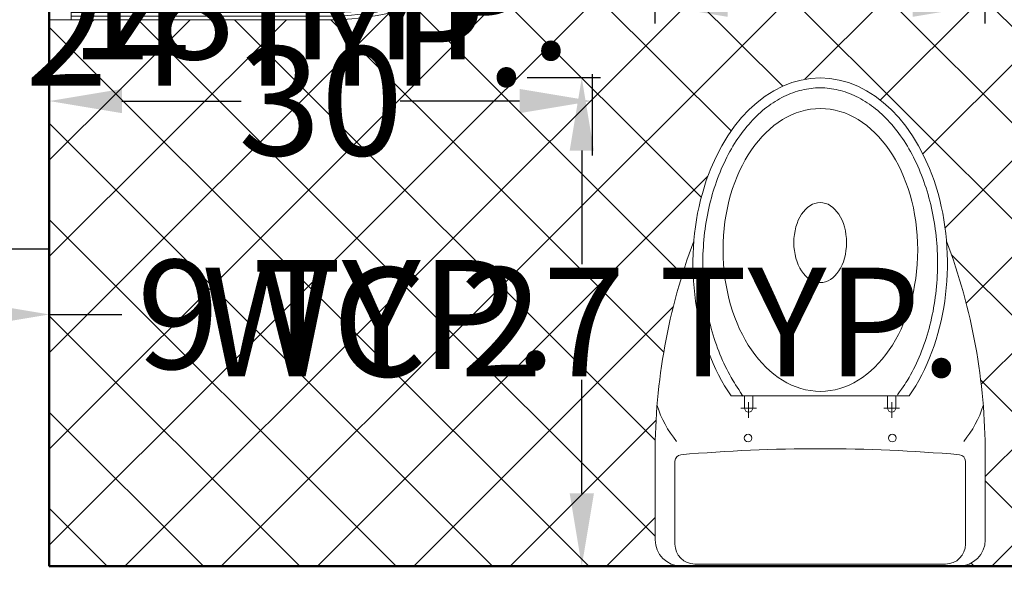
# Model space of a CAD drawing. Units: inches. Extents: x -466983 to 1020, y 324 to 318697.
# Tile 5 of 97: x 450 to 504, y 566 to 597. Entities that reach past the tile are written whole.
import ezdxf

# ---------------------------------------------------------------- set-up
doc = ezdxf.new("R2010")
doc.units = ezdxf.units.IN
doc.header["$MEASUREMENT"] = 0
for name, color, linetype, lineweight in [('A-ANNO-DIMS', 2, 'Continuous', 18), ('A-FLOR-FIXT', 9, 'Continuous', 18), ('A-FLOR-PATT', 252, 'Continuous', 13), ('A-GLAZ', 4, 'Continuous', 25), ('A-WALL', 7, 'Continuous', 50)]:
    doc.layers.add(name, color=color, linetype=linetype, lineweight=lineweight)
doc.styles.get("Standard").update_dxf_attribs({"font": 'arial.ttf'})
doc.dimstyles.get("Standard").update_dxf_attribs({"dimtxt": 6, "dimasz": 4, "dimexe": 3, "dimexo": 3, "dimgap": 0.09, "dimtad": 0, "dimtih": 1, "dimtoh": 1, "dimdec": 1, "dimzin": 0, "dimdsep": 46, "dimlunit": 3, "dimtxsty": 'Standard', "dimcen": 0.09, "dimadec": 0, "dimazin": 0, "dimtfac": 1, "dimtdec": 1, "dimtofl": 0, "dimtmove": 0, "dimatfit": 3, "dimfxl": 1, "dimtolj": 1, "dimtzin": 0, "dimarcsym": 0})

# ---------------------------------------------------------------- blocks, each defined once
blk = doc.blocks.new('Ventilator')
for p, q in [((1433.5927409432, 801.6799676286266), (1457.592740943201, 801.6799676286266)), ((1433.5927409432, 792.6799676286266), (1433.5927409432, 801.6799676286266)), ((1457.592740943201, 801.6799676286266), (1457.592740943201, 792.6799676286266)), ((1433.5927409432, 797.9799676286265), (1457.592740943201, 797.9799676286265)), ((1457.592740943201, 796.3799676286266), (1433.5927409432, 796.3799676286266)), ((1457.592740943201, 792.6799676286266), (1433.5927409432, 792.6799676286266))]:
    blk.add_line(p, q)
blk = doc.blocks.new('B1')
for p, q in [((0, 1300.000000000277), (693.3333333334303, 1300.000000000277)), ((0, 1.023182e-10), (0, 1300.000000000277)), ((52.00000000000727, 52.00000000000045), (52.00000000000727, 1300.000000000277)), ((52.00000000000727, 1291.33333333362), (693.3333333334303, 1291.33333333362)), ((52.00000000000727, 1282.666666666948), (693.3333333334303, 1282.666666666948)), ((0, 1248.000000000277), (693.3333333334303, 1248.000000000277)), ((21.99999999999818, 689.0000000001346), (21.99999999999818, 687.0000000001382)), ((140.3876720592416, 699.4289321882679), (154.4144116848583, 699.4289321882679)), ((208.8876720592416, 705.4289321882679), (153.4804125083301, 702.8756022550479)), ((1248.000000000174, 693.6609680139231), (1248.000000000174, 1.023182e-10)), ((1282.666666666846, 693.6609680139231), (1282.666666666846, 52.00000000010231)), ((1291.333333333514, 693.6609680139231), (1291.333333333517, 52.00000000010231)), ((1300.000000000182, 693.6609680139231), (1300.000000000182, 1.023182e-10)), ((21.99999999999818, 663.0000000001382), (21.99999999999818, 665.0000000001309)), ((140.3876720592416, 652.5710678120049), (154.4144116848583, 652.5710678120049)), ((208.8876720592416, 646.5710678120049), (153.5459520445456, 648.976381547378)), ((52.00000000001091, 52.00000000000045), (1300.000000000178, 52.00000000010231)), ((0, 4.547e-13), (1300.000000000182, 1.023182e-10))]:
    blk.add_line(p, q)
for points in [[(0, 775.000000000131), (0, 789.0000000001346), (8, 789.0000000001346)], [(8, 789.0000000001346), (8, 717.0000000001309)], [(8, 789.0000000001346), (27.99999999999818, 769.0000000001309), (27.99999999999818, 767.0000000001382)], [(0, 754.0000000001382), (0, 775.000000000131)], [(27.99999999999818, 767.0000000001382), (33.00000000000182, 767.0000000001382)], [(27.99999999999818, 767.0000000001382), (27.99999999999818, 753.0000000001345)], [(33.00000000000182, 767.0000000001382), (35, 769.0000000001309), (43, 769.0000000001309), (45.00000000000182, 767.0000000001382)], [(33.00000000000182, 767.0000000001382), (33.00000000000182, 753.0000000001345)], [(35, 765.0000000001345), (33.00000000000182, 762.0000000001346)], [(33.00000000000182, 758.0000000001346), (35, 756.0000000001346), (43, 756.0000000001346), (45.00000000000182, 758.0000000001346)], [(43, 769.0000000001309), (43, 765.0000000001345), (35, 765.0000000001345), (35, 769.0000000001309)], [(35, 756.0000000001346), (35, 753.0000000001345)], [(43, 765.0000000001345), (45.00000000000182, 763.0000000001382)], [(43, 756.0000000001346), (43, 753.0000000001345)], [(47, 767.0000000001382), (45.00000000000182, 767.0000000001382)], [(45.00000000000182, 767.0000000001382), (45.00000000000182, 753.0000000001345)], [(47, 739.0000000001382), (47, 767.0000000001382)], [(8, 717.0000000001309), (0, 717.0000000001309), (0, 754.0000000001382)], [(8, 717.0000000001309), (27.99999999999818, 737.0000000001346), (27.99999999999818, 739.0000000001382)], [(27.99999999999818, 739.0000000001382), (27.99999999999818, 753.0000000001345)], [(27.99999999999818, 739.0000000001382), (33.00000000000182, 739.0000000001382)], [(33.00000000000182, 739.0000000001382), (33.00000000000182, 753.0000000001345)], [(33.00000000000182, 748.0000000001382), (35, 750.0000000001346), (43, 750.0000000001346), (45.00000000000182, 748.0000000001382)], [(35, 741.0000000001346), (33.00000000000182, 744.0000000001345)], [(33.00000000000182, 739.0000000001382), (35, 737.0000000001346), (43, 737.0000000001346), (45.00000000000182, 739.0000000001382)], [(35, 750.0000000001346), (35, 753.0000000001345)], [(43, 737.0000000001346), (43, 741.0000000001346), (35, 741.0000000001346), (35, 737.0000000001346)], [(43, 750.0000000001346), (43, 753.0000000001345)], [(43, 741.0000000001346), (45.00000000000182, 743.0000000001346)], [(45.00000000000182, 739.0000000001382), (45.00000000000182, 753.0000000001345)], [(47, 739.0000000001382), (45.00000000000182, 739.0000000001382)], [(47, 728.0000000001345), (47, 739.0000000001382)], [(0, 687.0000000001382), (0, 699.0000000001382)], [(0, 699.0000000001382), (3, 699.0000000001382)], [(0, 665.0000000001309), (0, 687.0000000001382)], [(3, 699.0000000001382), (3, 676.0000000001346)], [(3, 699.0000000001382), (11, 690.0000000001382), (11, 687.0000000001382)], [(11, 687.0000000001382), (11, 676.0000000001346)], [(140.9999999999982, 687.0000000001382), (11, 687.0000000001382)], [(0, 653.0000000001309), (0, 665.0000000001309)], [(3, 653.0000000001309), (3, 676.0000000001346)], [(3, 653.0000000001309), (11, 662.000000000131), (11, 665.0000000001309)], [(11, 665.0000000001309), (11, 676.0000000001346)], [(140.9999999999982, 665.0000000001309), (11, 665.0000000001309)], [(0, 653.0000000001309), (3, 653.0000000001309)], [(133.9221670278657, 656.0563042479444), (133.0620831697051, 656.0563042479444)], [(7.999999999998181, 635.0000000001382), (0, 635.0000000001382), (0, 598.0000000001309)], [(7.999999999998181, 563.0000000001346), (7.999999999998181, 635.0000000001382)], [(7.999999999998181, 635.0000000001382), (27.99999999999818, 615.0000000001345), (27.99999999999818, 613.0000000001346)], [(27.99999999999818, 613.0000000001346), (27.99999999999818, 599.0000000001382)], [(27.99999999999818, 613.0000000001346), (33.00000000000182, 613.0000000001346)], [(33.00000000000182, 613.0000000001346), (35, 615.0000000001345), (42.99999999999818, 615.0000000001345), (45.00000000000182, 613.0000000001346)], [(33.00000000000182, 613.0000000001346), (33.00000000000182, 599.0000000001382)], [(42.99999999999818, 615.0000000001345), (42.99999999999818, 611.0000000001382), (35, 611.0000000001382), (35, 615.0000000001345)], [(45.00000000000182, 613.0000000001346), (45.00000000000182, 599.0000000001382)], [(47, 613.0000000001346), (45.00000000000182, 613.0000000001346)], [(47, 624.0000000001345), (47, 613.0000000001346)], [(47, 613.0000000001346), (47, 585.0000000001346)], [(0, 598.0000000001309), (0, 577.0000000001382)], [(27.99999999999818, 585.0000000001346), (27.99999999999818, 599.0000000001382)], [(35, 611.0000000001382), (33.00000000000182, 608.0000000001382)], [(33.00000000000182, 604.0000000001346), (35, 602.0000000001382), (42.99999999999818, 602.0000000001382), (45.00000000000182, 604.0000000001346)], [(33.00000000000182, 585.0000000001346), (33.00000000000182, 599.0000000001382)], [(33.00000000000182, 594.0000000001345), (35, 596.0000000001382), (42.99999999999818, 596.0000000001382), (45.00000000000182, 594.0000000001345)], [(35, 587.0000000001382), (33.00000000000182, 590.0000000001382)], [(35, 602.0000000001382), (35, 599.0000000001382)], [(35, 596.0000000001382), (35, 599.0000000001382)], [(42.99999999999818, 611.0000000001382), (45.00000000000182, 609.0000000001346)], [(42.99999999999818, 602.0000000001382), (42.99999999999818, 599.0000000001382)], [(42.99999999999818, 596.0000000001382), (42.99999999999818, 599.0000000001382)], [(45.00000000000182, 585.0000000001346), (45.00000000000182, 599.0000000001382)], [(0, 577.0000000001382), (0, 563.0000000001346), (7.999999999998181, 563.0000000001346)], [(7.999999999998181, 563.0000000001346), (27.99999999999818, 583.000000000131), (27.99999999999818, 585.0000000001346)], [(27.99999999999818, 585.0000000001346), (33.00000000000182, 585.0000000001346)], [(33.00000000000182, 585.0000000001346), (35, 583.000000000131), (42.99999999999818, 583.000000000131), (45.00000000000182, 585.0000000001346)], [(42.99999999999818, 583.000000000131), (42.99999999999818, 587.0000000001382), (35, 587.0000000001382), (35, 583.000000000131)], [(42.99999999999818, 587.0000000001382), (45.00000000000182, 589.0000000001309)], [(47, 585.0000000001346), (45.00000000000182, 585.0000000001346)]]:
    blk.add_lwpolyline(points)
blk.add_lwpolyline([(208.8876720592416, 646.5710678120049), (154.6376720593016, 648.9289321882679, -0.1383183006310921), (148.063043746286, 650.7831906028294, -0.0370381408635636), (145.578855038857, 652.5710678120049), (140.3876720592379, 652.5710678120049, -0.1665558057867227), (136.092755137337, 654.0425753596318, -0.0535717192020755), (133.4948936773198, 656.547585930646), (107, 654.0000000001382, 0.2625940722123521), (85, 631.0000000001346), (72, 580.0000000001419), (47, 580.0000000001419), (47, 585.0000000001346), (45.00000000000182, 585.0000000001346), (42.99999999999818, 583.0000000001346), (35, 583.0000000001346), (33.00000000000182, 585.0000000001346), (27.99999999999818, 585.0000000001346), (27.99999999999818, 583.0000000001346), (7.999999999998181, 563.0000000001382), (0, 563.0000000001382), (0, 577.0000000001418), (0, 598.0000000001346), (0, 635.0000000001418), (7.999999999998181, 635.0000000001418), (27.99999999999818, 615.0000000001382), (27.99999999999818, 613.0000000001346), (33.00000000000182, 613.0000000001346), (35, 615.0000000001382), (42.99999999999818, 615.0000000001382), (45.00000000000182, 613.0000000001346), (47, 613.0000000001346), (47, 624.0000000001382, 0.1247866838288863), (46, 648.0000000001382, 0.1501483781683498), (42.00000000000182, 654.0000000001382, -0.1384844099870248), (32.50754085593508, 665.0000000001345), (21.99999999999818, 665.0000000001345), (21.99999999999818, 663.0000000001382, -0.3003468456066685), (11, 662.3397459768711), (11, 662.0000000001346), (3, 653.0000000001345), (0, 653.0000000001345), (0, 665.0000000001345), (0, 687.0000000001382), (0, 699.0000000001418), (3, 699.0000000001418), (11, 690.0000000001382), (10.99999999999636, 689.6602540496569, -0.3003468456580443), (21.99999999999818, 689.0000000001346), (21.99999999999818, 687.0000000001382), (32.50754085593508, 687.0000000001382, -0.138484409987018), (42.00000000000182, 698.0000000001346, 0.1501483781683498), (46, 704.0000000001346, 0.1247866838288863), (47, 728.0000000001382), (47, 739.0000000001382), (45.00000000000182, 739.0000000001382), (43, 737.0000000001382), (35, 737.0000000001382), (33.00000000000182, 739.0000000001382), (27.99999999999818, 739.0000000001382), (27.99999999999818, 737.0000000001382), (8, 717.0000000001346), (0, 717.0000000001346), (0, 754.0000000001382), (0, 775.0000000001346), (0, 789.0000000001382), (8, 789.0000000001382), (27.99999999999818, 769.0000000001345), (27.99999999999818, 767.0000000001382), (33.00000000000182, 767.0000000001382), (35, 769.0000000001345), (43, 769.0000000001345), (45.00000000000182, 767.0000000001382), (47, 767.0000000001382), (47, 772.0000000001346), (72, 772.0000000001346), (85, 721.0000000001382, 0.2625940722123521), (107, 698.0000000001346), (133.494893670435, 695.4524140702815, -0.0535717192022979), (136.092755137337, 697.9574246406409, -0.1665558057868109), (140.3876720592416, 699.4289321882679), (145.7502000114491, 699.4289321882679, -0.0343443404771406), (148.063043746286, 701.07467377371, -0.1383183006298331), (154.6376720592416, 702.9289321882715), (208.8876720591488, 705.4289321882679, -0.1377032461334603), (216.0999264221609, 703.4042378869926, -0.1070360850488126), (223.0298076829695, 696.809397513447, -0.0808015121757586), (227.273223711496, 687.6931912444343, -0.0687078013104136), (228.8876720592398, 676.0000000001382, -0.0687078013104135), (227.273223711496, 664.3068087558385, -0.0808015121757595), (223.0298076829695, 655.1906024868258, -0.107036085048811), (216.0999264221609, 648.5957621132802, -0.1377032461317454)], format="xyb", close=True)
for points in [[(47, 767.0000000001382), (47, 772.0000000001309), (72, 772.0000000001309), (85, 721.0000000001382, 0.2625940722123521), (107, 698.0000000001346), (133.4948936704422, 695.4524140702887, -0.3591123035969264)], [(47, 734.0000000001346, -0.2052577019546359), (52, 726.0000000001309, -0.1374236490949136), (49, 701.0000000001346, -5.029096516974528)], [(47, 728.0000000001345, -0.1247866838288863), (46, 704.0000000001346, -0.1501483781683498), (42.00000000000182, 698.0000000001346, 0.138484409987018), (32.50754085593508, 687.0000000001382, 0.7633705308853952)], [(11, 688.0000000001346, -0.2034527507076884), (11.27314869702968, 688.6434964536201, -0.0971632324952149), (12.46446609406666, 689.4142135625043, -0.0541309211895364), (13.96123847455419, 689.8322469457524, -0.041071521782227), (15.99999999999818, 690.0000000001382, -0.041071521782232), (18.03876152544581, 689.8322469457524, -0.0541309211895581), (19.53553390593333, 689.4142135625043, -0.0971632324952149), (20.72685130297032, 688.6434964536201, -0.2034527507076884), (21, 688.0000000001346, -0.2034527507076693), (20.72685130297032, 687.3565035466526, -0.0379533313060429), (20.29672106629732, 687.0000000001382, -0.0541309211895384)], [(11.70327893370086, 687.0000000001382, -0.0379533313059558), (11.27314869702968, 687.3565035466526, -0.2034527507076722), (11, 688.0000000001346, -0.2034527507076884)], [(11.14357068821118, 689.7415727613479, -0.2958552022276962), (21.99999999999818, 689.0000000001346, -2.290285352134018)], [(106.0000000000018, 698.0000000001346), (73, 703.0000000001382, 0.3410628393219512), (44.19402075297876, 687.0000000001382, 0.987420997957196)], [(71.00000000000182, 698.0000000001346, 0.2653451188970793), (52.73167562087656, 687.0000000001382, 0.6855978624637613)], [(71.00000000000182, 698.0000000001346), (130.3767751999166, 690.0830966401517, -0.389881551935721)], [(109.0000000000018, 693.0000000001382, 0.3394066855219726), (103.0542662941007, 687.0000000001382)], [(105.3371881863113, 687.0000000001382, -0.2701562118716146), (110, 691.0000000001346), (129.6983785438242, 688.2641140912746, -0.3982822486971544)], [(106.0000000000018, 698.0000000001346), (132.9051195245556, 694.7054955685562, -0.3445125279727503)], [(129.2869436463206, 665.0799945585786, 0.0546118951167688), (131.5488372944073, 659.4332431739494, 0.1055200220071626), (136.092755137337, 654.0425753596318, 0.1665558057868128), (140.3876720592416, 652.5710678120049, 0.1665558057868108), (144.6825889811407, 654.0425753596318, 0.1055200220071628), (149.2265068240704, 659.4332431739494, 0.0682582856346859), (151.8562849435693, 666.5533485092964, 0.0544283700167335), (152.8876720592398, 676.0000000001346, 0.0544283700167333), (151.8562849435693, 685.4466514909764, 0.0682582856346864), (149.2265068240704, 692.5667568263307, 0.1055200220071624), (144.6825889811407, 697.9574246406409, 0.1665558057868127), (140.3876720592416, 699.4289321882679, 0.1665558057868109), (136.092755137337, 697.9574246406409, 0.1055200220071607), (131.5488372944073, 692.5667568263307, 0.0538660454735237), (129.3093729212014, 687.0000000001382, 0.0544283700167342)], [(140.9999999999982, 665.0000000001309, 0.130158640187584), (143.919967274478, 665.7732172227988, 0.1064685849763611), (146.6568542494933, 668.2218254070867, 0.0842476149744631), (148.3593095850538, 671.6519929664936, 0.0732806852421333), (149, 676.0000000001346, 0.0732806852421325), (148.3593095850538, 680.3480070337755, 0.0842476149744645), (146.6568542494933, 683.7781745931861, 0.1064685849763632), (143.919967274478, 686.226782777474, 0.1301586401875921), (140.9999999999982, 687.0000000001382, 0.1301586401875932)], [(141.6455361051521, 652.6849517968694, 0.0451764077839428), (142.9034001510663, 652.5710678120049, 0.1665558057868108), (147.1983170729654, 654.0425753596318, 0.1055200220071628), (151.7422349158969, 659.4332431739494, 0.0682582856346859), (154.3720130353958, 666.5533485092964, 0.0544283700167335), (155.4034001510663, 676.0000000001346, 0.0544283700167333), (154.3720130353958, 685.4466514909764, 0.0682582856346864), (151.7422349158969, 692.5667568263307, 0.1055200220071624), (147.1983170729654, 697.9574246406409, 0.1665558057868127), (142.9034001510663, 699.4289321882679, 0.0451764077839423), (141.6455361051521, 699.315048203407, 0.1055200220071607)], [(145.5788550388533, 652.5710678120049, 0.0370381408635636), (148.063043746286, 650.7831906028294, 0.1383183006298338), (154.6376720592416, 648.9289321882679, 0.138318300629834), (161.2123003721917, 650.7831906028294, 0.1070627939593127), (167.5423708158942, 656.8370490962297, 0.0805227312927088), (171.4136097265637, 665.1966168081926, 0.0683531574638633), (172.8876720592398, 675.9289321882679, 0.0683531574638646), (171.4136097265637, 686.6612475683432, 0.0805227312927094), (167.5423708158942, 695.0208152803061, 0.1070627939593105), (161.2123003721917, 701.07467377371, 0.1383183006298341), (154.6376720592416, 702.9289321882715, 0.1383183006298331), (148.063043746286, 701.07467377371, 0.0343443404771406), (145.7502000114491, 699.4289321882679, 0.0805227312927093)], [(154.4144116848583, 652.5710678120049, 0.1665558057868108), (158.7093286067611, 654.0425753596318, 0.1055200220071628), (163.2532464496908, 659.4332431739494, 0.0682582856346859), (165.8830245691897, 666.5533485092964, 0.0544283700167335), (166.9144116848601, 676.0000000001346, 0.0544283700167333), (165.8830245691897, 685.4466514909764, 0.0682582856346864), (163.2532464496908, 692.5667568263307, 0.1055200220071624), (158.7093286067611, 697.9574246406409, 0.1665558057868127), (154.4144116848583, 699.4289321882679, 0.1665558057868109)], [(207.6853336958775, 646.6233249695179, 0.0217212157548433), (208.8876720592416, 646.5710678120049, 0.1377032461317454), (216.0999264221609, 648.5957621132802, 0.107036085048811), (223.0298076829695, 655.1906024868258, 0.0808015121757595), (227.273223711496, 664.3068087558385, 0.0687078013104135), (228.8876720592398, 676.0000000001346, 0.0687078013104136), (227.273223711496, 687.6931912444343, 0.0808015121757586), (223.0298076829695, 696.809397513447, 0.1070360850488126), (216.0999264221609, 703.4042378869926, 0.1377032461317515), (208.8876720592416, 705.4289321882679, 0.0115815460008583), (208.2459469633304, 705.4140658567775, 0.1070360850488107)], [(11, 664.0000000001346, 0.2034527507076884), (11.27314869702968, 663.356503546649, 0.0971632324952149), (12.46446609406666, 662.5857864377649, 0.0541309211895364), (13.96123847455419, 662.1677530545167, 0.041071521782227), (15.99999999999818, 662.000000000131, 0.041071521782232), (18.03876152544581, 662.1677530545167, 0.0541309211895581), (19.53553390593333, 662.5857864377649, 0.0971632324952149), (20.72685130297032, 663.356503546649, 0.2034527507076884), (21, 664.0000000001346, 0.2034527507076693), (20.72685130297032, 664.6434964536202, 0.0379533313062782), (20.29672106629369, 665.0000000001309, 0.0541309211895384)], [(11.70327893370449, 665.0000000001309, 0.0379533313061481), (11.27314869702968, 664.6434964536202, 0.2034527507076722), (11, 664.0000000001346, 0.2034527507076884)], [(11.14357068821118, 662.2584272389249, 0.2958552022276962), (21.99999999999818, 663.0000000001382, 2.290285352134018)], [(47, 624.0000000001345, 0.1247866838288863), (46, 648.0000000001382, 0.1501483781683498), (42.00000000000182, 654.0000000001382, -0.1384844099870248), (32.50754085593508, 665.0000000001309, -0.7633705308853952)], [(106.0000000000018, 654.0000000001382), (73, 649.0000000001345, -0.341062839321959), (44.19402075297876, 665.0000000001309, -0.987420997957196)], [(71.00000000000182, 654.0000000001382, -0.2653451188970914), (52.73167562087656, 665.0000000001309, -0.6855978624637613)], [(71.00000000000182, 654.0000000001382), (130.3767751999166, 661.9169033601211, 0.389881551935721)], [(109.0000000000018, 659.0000000001309, -0.3394066855220244), (103.0542662941007, 665.0000000001309)], [(105.3371881863113, 665.0000000001309, 0.2701562118716416), (110, 661.0000000001345), (129.6983785438278, 663.7358859089982, 0.3982822486971544)], [(47, 585.0000000001346), (47, 580.0000000001382), (72, 580.0000000001382), (85, 631.0000000001346, -0.2625940722123521), (107, 654.0000000001382), (132.4235230446356, 656.4445695236572, 0.3591123035969264)], [(47, 618.0000000001346, 0.2052577019546359), (52, 626.0000000001382, 0.1374236490949136), (49, 651.0000000001382, 5.029096516974528)], [(106.0000000000018, 654.0000000001382), (132.9051195245556, 657.2945044317166, 0.3445125279727503)]]:
    blk.add_lwpolyline(points, format="xyb")
blk.add_circle((182.931355266388, 149.5974501754249), 47.86997641275996)
for centre, radius, start, end in [((672.5535632588981, 672.5422464127919), 627.8017452838134, 1.92774542086775, 88.10320593202876), ((672.5535632588981, 672.5422464127919), 610.4684119504776, 1.92774542086775, 88.10320593202876), ((672.5535632588981, 672.5422464127919), 619.1350786171454, 1.92774542086775, 88.10320593202876), ((672.5535632588981, 672.5422464127919), 575.801745283806, 1.92774542086775, 88.10320593202876), ((84, 676.0000000001346), 19, 35.37654015188604, 144.6234598481139), ((84, 676.0000000001346), 12.00000000000001, 66.44353569094163, 113.5564643090584), ((120.8125, 676.1250000001309), 12.8131097415889, 112.0608994672246, 121.9251013585072), ((123.9999999999982, 676.0000000001346), 13, 64.79528984039216, 122.2042275039623), ((84, 676.0000000001346), 19, 215.376540151886, 324.623459848114), ((84, 676.0000000001346), 12.00000000000001, 246.4435356909416, 293.5564643090584), ((120.8125, 675.8750000001382), 12.8131097415889, 238.0748986414927, 247.9391005327754), ((123.9999999999982, 676.0000000001346), 13, 237.7957724960376, 295.2047101596079)]:
    blk.add_arc(centre, radius, start, end)
blk = doc.blocks.new('A$C005B7AE8')
for p, q in [((0.4599999173160541, 0.7399999669141835), (0.0399999173159813, 0.7399999669141835)), ((0.439999917316527, 0.7369231961274636), (0.0599999173164179, 0.7369231961274636)), ((0.0299999173166725, 0.7069231961286278), (0.029999917315763, 0.5811477270617617)), ((0.4699999173162724, 0.7069231961286278), (0.4699999173162724, 0.5811477270617617)), ((-8.26839823e-08, 0.6999999669133103), (-8.26839823e-08, 0.5690287834004267)), ((0.4999999173160177, 0.6999999669133103), (0.4999999173160177, 0.5690287833785987)), ((0.1415172819179133, 0.4916755243175431), (0.1415172819179133, 0.5154492432702682)), ((0.3584825527150315, 0.4916755243175431), (0.3584825527150315, 0.5154492432702682)), ((0.1298495880610062, 0.5003783992360696), (0.1533971911394474, 0.5003783992360696)), ((0.135565754210802, 0.4819999669125537), (0.135565754210802, 0.5011511907214299)), ((0.1478168830781215, 0.5011511907214299), (0.1478168830781215, 0.4819999669125537)), ((0.3701502465710291, 0.5003783992360696), (0.3466026434934974, 0.5003783992360696)), ((0.3521829515548234, 0.5011511907214299), (0.3521829515548234, 0.4819999669125537)), ((0.3644340804221429, 0.4819999669125537), (0.3644340804221429, 0.5011511907214299)), ((0.3846918195813487, 0.4819999669125537), (0.1153080150515962, 0.4819999669125537))]:
    blk.add_line(p, q)
for centre in [(0.1407590817070741, 0.546016981927096), (0.3592407529249613, 0.546016981927096)]:
    blk.add_circle(centre, 0.0058207128015492)
for centre, radius, start, end in [((0.0399999173159813, 0.6999999669133103), 0.04, 90, 180), ((0.0599999173164179, 0.7069231961286278), 0.03, 90, 180), ((0.439999917316527, 0.7069231961286278), 0.03, 0, 90), ((0.4599999173160541, 0.6999999669133103), 0.04, 0, 90), ((0.9162347733818023, 0.5697843573143473), 0.9162351676084766, 179.9527510438183, 200.6123382500767), ((0.0399999173159813, 0.5811477270617617), 0.01, 180, 265.0114580301616), ((0.2499999173160177, 2.986999966909934), 2.424999999999394, 265.0114580301616, 274.9885419698384), ((-0.4162349387497671, 0.5697843573143473), 0.9162351676084766, 339.3876617499233, 0.0472489561816761), ((0.4599999173160541, 0.5811477270617617), 0.01, 274.9885419698384, 0), ((0.1538218116911594, 0.4497837234594045), 0.1578971577643038, 140.181504794802, 162.8477667450203), ((0.346178022940876, 0.4497837234594045), 0.1578971577643038, 17.15223325497964, 39.81849520519793), ((0.141691318644007, 0.5005983719747747), 0.0061504591858251, 5.156848388262675, 174.8431516117373), ((0.3583085159880284, 0.5005983719747747), 0.0061504591858251, 5.156848388262675, 174.8431516117373)]:
    blk.add_arc(centre, radius, start, end)
blk.add_ellipse((0.2499999173160177, 0.2809999669116223), major_axis=(4.3e-15, -0.2809999999999999), ratio=0.6859192225533541, start_param=3.915332106759934, end_param=8.65103850759918)
for centre, major_axis, ratio in [((0.2497273054386824, 0.2607283879333408), (4.6e-15, -0.2143896387416461), 0.687861093389952), ((0.2499999173160177, 0.2495750337038771), (4e-16, -0.0607231097518234), 0.6571642650459009)]:
    blk.add_ellipse(centre, major_axis=major_axis, ratio=ratio)
blk.add_open_spline([(0.1330304284401791, 0.4805691871661111), (0.123297561966865, 0.467275065217109), (0.1192040598116364, 0.4608387557527749), (0.1089923119561718, 0.4430896997000673), (0.103240873932009, 0.4312752909245319), (0.0930943572666365, 0.4063656141879619), (0.0886993987696769, 0.3932708291395102), (0.0814055876480779, 0.3661625228414778), (0.0785067868491751, 0.352149423713854), (0.0742960000825406, 0.3235936370911077), (0.0729840366493591, 0.3090513401839416), (0.0719875980385041, 0.2798412472329801), (0.0723031276866095, 0.2651738304266473), (0.0745519352649353, 0.2361210512899561), (0.076485202062031, 0.2217360707581975), (0.0819094268572371, 0.1936478195857489), (0.0854003532995194, 0.1799449487807578), (0.0938301373234936, 0.1536010168056237), (0.0987689237617815, 0.1409603975334903), (0.1099364044266622, 0.1170889910499682), (0.116164929732804, 0.1058587174047716), (0.1297089136187424, 0.0851097239210503), (0.1370239707930523, 0.0755915829504375), (0.152501027386279, 0.0585057705757208), (0.1606621934961367, 0.0509385682526045), (0.1775722209031301, 0.0379140469667618), (0.1863198251348876, 0.0324565718765371), (0.2041561746218576, 0.023724375780148), (0.2132440667546689, 0.0204483489505947), (0.2315630702087219, 0.0160859502211679), (0.2407950771003016, 0.01499791808601), (0.259256859623747, 0.0150020215223776), (0.2684887415816775, 0.0160941591893789), (0.2868071874390807, 0.0204647859718534), (0.2958946431490403, 0.0237449365959037), (0.3137296967424845, 0.0324853214769974), (0.3224764393571604, 0.0379468595056096), (0.3393842548493922, 0.0509792925877264), (0.3475440710253679, 0.058550341942464), (0.3630179485271583, 0.0756434699942474), (0.3703311774997928, 0.0851650790282293), (0.3838710834670564, 0.1059204943594523), (0.3900973596782933, 0.1171537218178855), (0.4012600005589775, 0.1410304195233039), (0.4061961965880983, 0.1536733763350639), (0.4146205471060967, 0.1800212940433994), (0.4181086305634381, 0.1937258131365524), (0.423527009337704, 0.2218166234742966), (0.425457273147913, 0.2362025149268447), (0.4277000090169168, 0.2652563529190957), (0.4280124699726003, 0.2799239176820265), (0.427009923148944, 0.3091335394783528), (0.4256949202253964, 0.3236752172670094), (0.4214781782784485, 0.3522290158871328), (0.4185764618305257, 0.3662407460942632), (0.4112770365782126, 0.3933456040758756), (0.406879379678685, 0.4064383096483653), (0.3967277738520352, 0.4313431800474064), (0.3909739452683425, 0.4431548618158559), (0.380770586511062, 0.4608783582370961), (0.376689084062491, 0.467293849651469), (0.3673029200963356, 0.4823032274071011)], degree=3, knots=[3.915332106759953, 3.915332106759953, 3.915332106759953, 3.915332106759953, 4.014440589322762, 4.014440589322762, 4.176504673233075, 4.176504673233075, 4.338568757143389, 4.338568757143389, 4.500632841053702, 4.500632841053702, 4.662696924964015, 4.662696924964015, 4.824761008874329, 4.824761008874329, 4.986825092784642, 4.986825092784642, 5.148889176694956, 5.148889176694956, 5.310953260605269, 5.310953260605269, 5.473017344515582, 5.473017344515582, 5.635081428425896, 5.635081428425896, 5.797145512336209, 5.797145512336209, 5.959209596246522, 5.959209596246522, 6.121273680156836, 6.121273680156836, 6.283337764067149, 6.283337764067149, 6.445401847977462, 6.445401847977462, 6.607465931887776, 6.607465931887776, 6.769530015798089, 6.769530015798089, 6.931594099708402, 6.931594099708402, 7.093658183618716, 7.093658183618716, 7.255722267529029, 7.255722267529029, 7.417786351439342, 7.417786351439342, 7.579850435349656, 7.579850435349656, 7.741914519259969, 7.741914519259969, 7.903978603170283, 7.903978603170283, 8.066042687080596, 8.066042687080596, 8.22810677099091, 8.22810677099091, 8.390170854901225, 8.390170854901225, 8.552234938811539, 8.552234938811539, 8.651038507599205, 8.651038507599205, 8.651038507599205, 8.651038507599205])
blk = doc.blocks.new('*D61')
at = {"layer": 'A-ANNO-DIMS', "color": 0, "lineweight": -2, "transparency": 16777216}
for p, q in [((439.8056775209044, 608.403511460552), (436.2056775209045, 608.403511460552)), ((439.2056775209045, 604.403511460552), (439.2056775209045, 599.5978770812881)), ((439.2056775209045, 588.4035114605508), (439.2056775209045, 593.2091458398146)), ((439.8056775209044, 584.4035114605508), (436.2056775209045, 584.4035114605508))]:
    blk.add_line(p, q, dxfattribs=at)
at = {"layer": 'A-ANNO-DIMS', "color": 0, "transparency": 16777216}
for points in [[(438.5390108542378, 604.403511460552), (439.8723441875712, 604.403511460552), (439.2056775209045, 608.403511460552)], [(438.5390108542378, 588.4035114605508), (439.8723441875712, 588.4035114605508), (439.2056775209045, 584.4035114605508)]]:
    blk.add_solid(points, dxfattribs=at)
at = {"layer": 'Defpoints', "color": 0, "transparency": 16777216}
for p in [(442.8056775209045, 608.403511460552), (439.2056775209045, 584.4035114605508), (442.8056775209045, 584.4035114605508)]:
    blk.add_point(p, dxfattribs=at)
at = {"layer": 'A-ANNO-DIMS', "color": 0, "transparency": 16777216, "insert": (439.2056775209046, 596.403511460551), "char_height": 6, "attachment_point": 5}
blk.add_mtext('\\A1;VENTILATOR 24 TYP.', dxfattribs=at)
blk = doc.blocks.new('*D62')
at = {"layer": 'A-ANNO-DIMS', "color": 0, "lineweight": -2, "transparency": 16777216}
for p, q in [((442.8056775209042, 581.4035114605506), (442.8056775209042, 577.8035114605505)), ((451.8056775209043, 581.4035114605506), (451.8056775209043, 577.8035114605505)), ((446.8056775209042, 580.8035114605505), (447.8056775209043, 580.8035114605505)), ((451.8056775209043, 580.8035114605505), (455.8056775209043, 580.8035114605505))]:
    blk.add_line(p, q, dxfattribs=at)
at = {"layer": 'A-ANNO-DIMS', "color": 0, "transparency": 16777216}
for points in [[(446.8056775209042, 581.470178127217), (446.8056775209042, 580.1368447938838), (442.8056775209042, 580.8035114605505)], [(447.8056775209043, 581.470178127217), (447.8056775209043, 580.1368447938838), (451.8056775209043, 580.8035114605505)]]:
    blk.add_solid(points, dxfattribs=at)
at = {"layer": 'Defpoints', "color": 0, "transparency": 16777216}
for p in [(442.8056775209042, 584.4035114605506), (451.8056775209043, 584.4035114605506), (451.8056775209043, 580.8035114605505)]:
    blk.add_point(p, dxfattribs=at)
at = {"layer": 'A-ANNO-DIMS', "color": 0, "transparency": 16777216, "insert": (468.1678466887078, 580.8035114605505), "char_height": 6, "attachment_point": 5}
blk.add_mtext('\\A1;9 TYP.', dxfattribs=at)
blk = doc.blocks.new('*D75')
at = {"layer": 'A-ANNO-DIMS', "color": 0, "lineweight": -2, "transparency": 16777216}
for p, q in [((448.8056775209043, 626.937732818422), (444.3217849538132, 626.937732818422)), ((447.3217849538133, 622.937732818422), (447.3217849538133, 615.1878362669078)), ((447.3217849538133, 601.0451157044797), (447.3217849538133, 608.7950122559939)), ((448.8056775209043, 597.0451157044797), (444.3217849538132, 597.0451157044797))]:
    blk.add_line(p, q, dxfattribs=at)
at = {"layer": 'A-ANNO-DIMS', "color": 0, "transparency": 16777216}
for points in [[(446.6551182871466, 622.937732818422), (447.9884516204799, 622.937732818422), (447.3217849538133, 626.937732818422)], [(446.6551182871466, 601.0451157044797), (447.9884516204799, 601.0451157044797), (447.3217849538133, 597.0451157044797)]]:
    blk.add_solid(points, dxfattribs=at)
at = {"layer": 'Defpoints', "color": 0, "transparency": 16777216}
for p in [(451.8056775209043, 626.937732818422), (447.3217849538133, 597.0451157044797), (451.8056775209043, 597.0451157044797)]:
    blk.add_point(p, dxfattribs=at)
at = {"layer": 'A-ANNO-DIMS', "color": 0, "transparency": 16777216, "insert": (447.3217849538133, 611.9914242614506), "char_height": 6, "attachment_point": 5}
blk.add_mtext('\\A1;SHOWER TRAY 30', dxfattribs=at)
blk = doc.blocks.new('*D76')
at = {"layer": 'A-ANNO-DIMS', "color": 0, "lineweight": -2, "transparency": 16777216}
for p, q in [((451.8056775209041, 594.0451157044795), (451.8056775209041, 589.561223137388)), ((481.6982946348461, 594.0451157044795), (481.6982946348461, 589.561223137388)), ((455.8056775209041, 592.5612231373881), (462.3768564735095, 592.5612231373881)), ((477.6982946348461, 592.5612231373881), (471.1271156822407, 592.5612231373881))]:
    blk.add_line(p, q, dxfattribs=at)
at = {"layer": 'A-ANNO-DIMS', "color": 0, "transparency": 16777216}
for points in [[(455.8056775209041, 593.2278898040546), (455.8056775209041, 591.8945564707215), (451.8056775209041, 592.5612231373881)], [(477.6982946348461, 593.2278898040546), (477.6982946348461, 591.8945564707215), (481.6982946348461, 592.5612231373881)]]:
    blk.add_solid(points, dxfattribs=at)
at = {"layer": 'Defpoints', "color": 0, "transparency": 16777216}
for p in [(451.8056775209041, 597.0451157044794), (481.6982946348461, 597.0451157044794), (481.6982946348461, 592.5612231373881)]:
    blk.add_point(p, dxfattribs=at)
at = {"layer": 'A-ANNO-DIMS', "color": 0, "transparency": 16777216, "insert": (466.7519860778751, 592.5612231373881), "char_height": 6, "attachment_point": 5}
blk.add_mtext('\\A1;30', dxfattribs=at)
blk = doc.blocks.new('*D77')
at = {"layer": 'A-ANNO-DIMS', "color": 0, "lineweight": -2, "transparency": 16777216}
for p, q in [((482.1546064346701, 593.8335263890428), (478.1202373990772, 593.8335263890428)), ((481.1202373990773, 589.8335263890428), (481.1202373990773, 583.5779488397488)), ((481.1202373990773, 570.9377328184221), (481.1202373990773, 577.193310367716)), ((482.1546064346701, 566.9377328184221), (478.1202373990772, 566.9377328184221))]:
    blk.add_line(p, q, dxfattribs=at)
at = {"layer": 'A-ANNO-DIMS', "color": 0, "transparency": 16777216}
for points in [[(480.4535707324105, 589.8335263890428), (481.786904065744, 589.8335263890428), (481.1202373990773, 593.8335263890428)], [(480.4535707324105, 570.9377328184221), (481.786904065744, 570.9377328184221), (481.1202373990773, 566.9377328184221)]]:
    blk.add_solid(points, dxfattribs=at)
at = {"layer": 'Defpoints', "color": 0, "transparency": 16777216}
for p in [(485.1546064346701, 593.8335263890428), (481.1202373990773, 566.9377328184221), (485.1546064346701, 566.9377328184221)]:
    blk.add_point(p, dxfattribs=at)
at = {"layer": 'A-ANNO-DIMS', "color": 0, "transparency": 16777216, "insert": (481.1202373990773, 580.3856296037322), "char_height": 6, "attachment_point": 5}
blk.add_mtext('\\A1;WC 27 TYP.', dxfattribs=at)
blk = doc.blocks.new('*D78')
at = {"layer": 'A-ANNO-DIMS', "color": 0, "lineweight": -2, "transparency": 16777216}
for p, q in [((485.1546064346699, 596.8335263890426), (485.1546064346699, 600.8678954246358)), ((503.334059280452, 596.8335263890426), (503.334059280452, 600.8678954246358)), ((485.1546064346699, 597.8678954246357), (481.1546064346699, 597.8678954246357)), ((499.334059280452, 597.8678954246357), (489.1546064346699, 597.8678954246357))]:
    blk.add_line(p, q, dxfattribs=at)
at = {"layer": 'A-ANNO-DIMS', "color": 0, "transparency": 16777216}
for points in [[(489.1546064346699, 598.5345620913023), (489.1546064346699, 597.2012287579691), (485.1546064346699, 597.8678954246357)], [(499.334059280452, 598.5345620913023), (499.334059280452, 597.2012287579691), (503.334059280452, 597.8678954246357)]]:
    blk.add_solid(points, dxfattribs=at)
at = {"layer": 'Defpoints', "color": 0, "transparency": 16777216}
for p in [(485.1546064346699, 597.8678954246357), (485.1546064346699, 593.8335263890426), (503.334059280452, 593.8335263890426)]:
    blk.add_point(p, dxfattribs=at)
at = {"layer": 'A-ANNO-DIMS', "color": 0, "transparency": 16777216, "insert": (466.7440061618186, 597.8678954246357), "char_height": 6, "attachment_point": 5}
blk.add_mtext('\\A1;18 TYP.', dxfattribs=at)

msp = doc.modelspace()

# ---------------------------------------------------------------- hatches: boundary and pattern name
at = {"layer": 'A-FLOR-PATT', "transparency": 33554572}
h = msp.add_hatch(dxfattribs=at)
h.set_pattern_fill('ANSI37', color=256, scale=30)
h.set_pattern_definition([(45, (-1212.413693079869, -290.0350025265127), (-2.651650429449553, 2.651650429449553), []), (135, (-1212.413693079869, -290.0350025265127), (-2.651650429449553, -2.651650429449552), [])])
h.paths.add_polyline_path([(901.805677520904, 1075.937732818422), (900.6144036774049, 1075.937732818422), (900.6144036774049, 1065.385628316983), (899.390971271441, 1065.385628316983), (898.0910743401043, 1065.385628316983), (892.8355944880973, 1058.709752245277, -0.2583770168556315), (892.18750428989, 1058.350891982691), (879.9847834232776, 1058.350891982691, -0.2017697719240963), (879.438188978411, 1058.580825279484), (874.0812133730635, 1065.385628316983), (872.7813164417267, 1065.385628316983), (871.5578840357629, 1065.385628316983), (871.5578840357629, 1075.937732818422), (813.8056775209042, 1075.937732818422), (813.8056775209042, 1044.792233318721), (832.3947444543938, 1044.792233318721, -0.3947951267487684), (848.6601780212009, 1028.535584015862), (848.6601780212009, 1009.937732818421), (901.805677520904, 1009.937732818421), (901.805677520904, 1015.937732818421), (901.3056775209042, 1015.937732818421), (871.3056775209039, 1015.937732818421), (871.3056775209039, 1017.250232818421), (871.3344022102003, 1017.250232818421, -0.4014527144963572), (901.3056775209042, 1045.937732818421), (901.805677520904, 1045.937732818421)])
edge = h.paths.add_edge_path(flags=16)
edge.add_line((847.7730719745084, 1068.948588737025), (847.7730719745069, 1073.708823774771))
edge.add_arc((849.2268986539951, 1073.708823774771), 1.453826679487974, 90, 180, ccw=False)
edge.add_line((849.2268986539951, 1075.162650454259), (864.4920787886183, 1075.162650454259))
edge.add_arc((864.4920787886213, 1073.708823774771), 1.453826679487974, 0, 90.00000000012102, ccw=False)
edge.add_line((865.9459054681093, 1073.708823774771), (865.9459054681081, 1069.00351244647))
edge.add_arc((832.6447385074767, 1068.976050591752), 33.30117828385809, -20.61233806670998, 0.04724903539101888, ccw=False)
edge.add_ellipse((856.8594887213083, 1058.479989307073), major_axis=(-2.091e-13, 10.21313242340307), ratio=0.6859192225533502, start_angle=100.00884331843292, end_angle=259.9911566815624, ccw=False)
edge.add_arc((881.0742389351396, 1068.976050591752), 33.30117828385809, 180.0472490354062, 200.6123380667097, ccw=False)
h.paths.add_polyline_path([(853.145578187156, 1066.481532374271), (853.145578187156, 1066.453444752512), (853.1463399851561, 1066.453444752512, 0.4331071439582673), (852.9166149812349, 1066.684892837266), (852.9166149812349, 1066.453444752512), (853.145578187156, 1066.453444752512), (853.145578187156, 1066.481532374489), (853.088019486549, 1066.612171966583, 0.6979386910037918), (852.699540939094, 1066.453444752512), (852.7003027371272, 1066.453444752512), (852.7003027371272, 1066.481532374489), (852.9166149812349, 1067.001204630995), (852.9166149812349, 1066.684892837266, -0.3962543063594317)], flags=0)
h.paths.add_polyline_path([(861.0186747055222, 1066.481532374271), (861.0186747055222, 1066.453444752512), (861.0194365035225, 1066.453444752512, 0.4164039232557909), (860.8023624614146, 1066.684892837265), (860.8023624614146, 1066.453444752512), (861.0186747055222, 1066.453444752512), (861.0186747055222, 1066.481532374489), (860.9671752720659, 1066.605255499379, 0.7133437187663149), (860.5726374574602, 1066.453444752512), (860.5733992554934, 1066.453444752512), (860.5733992554934, 1066.481532374489), (860.8023624614146, 1067.001204630995), (860.8023624614146, 1066.684892837265, -0.3799725304814568)], flags=0)
edge = h.paths.add_edge_path(flags=0)
edge.add_spline(control_points=[(861.1298377106021, 1065.785468371534), (861.4660965533383, 1065.247811229462), (861.613385559155, 1065.016139861057), (861.9832837951076, 1064.373617117607), (862.1924105327118, 1063.944313665492), (862.5613774174725, 1063.039129539609), (862.7212131906668, 1062.56326642291), (862.9865156700853, 1061.578122280975), (863.0919804897928, 1061.068856600952), (863.2452407883674, 1060.031049745086), (863.293035446714, 1059.502522766744), (863.3294736797056, 1058.440879580113), (863.3181170778639, 1057.907777155726), (863.2366033468288, 1056.85179603536), (863.1664466211855, 1056.328931215311), (862.9695120306455, 1055.307951977375), (862.8427353108815, 1054.809852090196), (862.5365466723708, 1053.852219447362), (862.3571373353129, 1053.392702749349), (861.9514237071658, 1052.524888245794), (861.7251255454219, 1052.116609101398), (861.2330086320977, 1051.362239687588), (860.9672044472572, 1051.016170456457), (860.4047960485765, 1050.394909316517), (860.1082220871676, 1050.119734477926), (859.493696255806, 1049.64606200509), (859.1757900615103, 1049.447558762665), (858.5275631429041, 1049.129883644436), (858.197273503909, 1049.010664382187), (857.5314773710529, 1048.851811036626), (857.1959384637446, 1048.812116564677), (856.5249326641573, 1048.811967422545), (856.1893892160524, 1048.851512676201), (855.5235728169741, 1049.010066967686), (855.1932673158994, 1049.129136347874), (854.5449932971788, 1049.446513839261), (854.2270557868354, 1049.644869411481), (853.6124495619564, 1050.118254324803), (853.3158265363004, 1050.393289340464), (852.7533025914207, 1051.014284587242), (852.487431959371, 1051.360227769297), (851.9951668313728, 1052.114363776776), (851.7687869247744, 1052.522535562859), (851.3628973914427, 1053.390157753425), (851.1833939042357, 1053.849589492002), (850.8770077813263, 1054.807077270704), (850.7501277313783, 1055.30511724975), (850.5529806633081, 1056.326003473117), (850.4827147921034, 1056.848835185142), (850.4009803807432, 1057.904777820697), (850.3895122452288, 1058.437874867502), (850.425728471152, 1059.499535178563), (850.4734126571939, 1060.02808465918), (850.6264565107679, 1061.065963770327), (850.7318153592672, 1061.575279204679), (850.9969137893603, 1062.560548677974), (851.1566514873134, 1063.036487374614), (851.525433403113, 1063.94184619004), (851.7344732542367, 1064.371248757046), (852.1056260411488, 1065.016350037675), (852.2544071072941, 1065.250281998093), (852.608154630964, 1065.733465727338)], knot_values=[3.915332106759953, 3.915332106759953, 3.915332106759953, 3.915332106759953, 4.013467662305501, 4.013467662305501, 4.175531746215815, 4.175531746215815, 4.337595830126129, 4.337595830126129, 4.499659914036444, 4.499659914036444, 4.661723997946757, 4.661723997946757, 4.82378808185707, 4.82378808185707, 4.985852165767384, 4.985852165767384, 5.147916249677697, 5.147916249677697, 5.30998033358801, 5.30998033358801, 5.472044417498324, 5.472044417498324, 5.634108501408637, 5.634108501408637, 5.79617258531895, 5.79617258531895, 5.958236669229264, 5.958236669229264, 6.120300753139577, 6.120300753139577, 6.282364837049891, 6.282364837049891, 6.444428920960204, 6.444428920960204, 6.606493004870517, 6.606493004870517, 6.768557088780831, 6.768557088780831, 6.930621172691144, 6.930621172691144, 7.092685256601457, 7.092685256601457, 7.254749340511771, 7.254749340511771, 7.416813424422084, 7.416813424422084, 7.578877508332397, 7.578877508332397, 7.740941592242711, 7.740941592242711, 7.903005676153024, 7.903005676153024, 8.065069760063338, 8.065069760063338, 8.22713384397365, 8.22713384397365, 8.389197927883965, 8.389197927883965, 8.551262011794279, 8.551262011794279, 8.650370494357087, 8.650370494357087, 8.650370494357087, 8.650370494357087], degree=3, periodic=0)
edge.add_line((852.6421178657537, 1065.785468371534), (861.1298377106024, 1065.785468371534))
edge = h.paths.add_edge_path(flags=0)
edge.add_ellipse((856.8495804607978, 1057.743205248224), major_axis=(-3.1e-13, 7.792134415209829), ratio=0.6878610933899516, start_angle=0, end_angle=360)
h.paths.add_polyline_path([(848.8634419841151, 1069.389059844444), (848.863441984139, 1073.960453158315, -0.4142135623709757), (849.9538119937549, 1075.050823167924), (863.765165448898, 1075.050823167924, -0.4142135623721942), (864.8555354585106, 1073.960453158308), (864.8555354584933, 1069.389059844444, -0.3889362887010341), (864.5236837164459, 1069.026979909221, -0.0435607626104464), (849.19529372618, 1069.02697990933, -0.3889362886276668)], flags=0)
h.paths.add_polyline_path([(853.1006153779753, 1068.112209480768, -1), (852.677499999749, 1068.112209480768, -1)], flags=0)
edge = h.paths.add_edge_path(flags=0)
edge.add_ellipse((856.8594887213083, 1057.33782914961), major_axis=(7.74e-14, 2.20702192546696), ratio=0.6571642650458812, start_angle=0, end_angle=360)
h.paths.add_polyline_path([(861.0414774428674, 1068.112209480768, -1), (860.6183620646412, 1068.112209480768, -1)], flags=0)
edge = h.paths.add_edge_path()
edge.add_line((573.9536545579417, 1057.341203598636), (573.9536545579417, 1075.937732818422))
edge.add_line((573.9536545579417, 1075.937732818422), (558.7307922536265, 1075.937732818422))
edge.add_line((558.7307922536265, 1075.937732818422), (558.7307922536265, 1065.385628316983))
edge.add_line((558.7307922536265, 1065.385628316983), (557.5073598476627, 1065.385628316983))
edge.add_line((557.5073598476627, 1065.385628316983), (556.207462916326, 1065.385628316983))
edge.add_line((556.207462916326, 1065.385628316983), (550.9519830643189, 1058.709752245277))
edge.add_arc((550.3038928661116, 1059.115537236419), 0.7646452537275144, 270, 327.94831933647396, ccw=False)
edge.add_line((550.3038928661116, 1058.350891982691), (538.1011719994992, 1058.350891982691))
edge.add_arc((538.1011719994992, 1059.115537236419), 0.7646452537275137, 224.3704013916024, 270, ccw=False)
edge.add_line((537.5545775546327, 1058.580825279484), (532.1976019492852, 1065.385628316983))
edge.add_line((532.1976019492852, 1065.385628316983), (530.8977050179485, 1065.385628316983))
edge.add_line((530.8977050179485, 1065.385628316983), (529.6742726119846, 1065.385628316983))
edge.add_line((529.6742726119846, 1065.385628316983), (529.6742726119846, 1075.937732818422))
edge.add_line((529.6742726119846, 1075.937732818422), (520.8056775209042, 1075.937732818422))
edge.add_line((520.8056775209042, 1075.937732818422), (520.8056775209042, 1045.937732818422))
edge.add_line((520.8056775209042, 1045.937732818422), (521.3056775209044, 1045.937732818422))
edge.add_arc((521.3056775209042, 1015.937732818422), 30.00000000000023, 2.507490703587223, 89.99999999999977, ccw=False)
edge.add_line((551.2769528316082, 1017.250232818422), (551.3056775209045, 1017.250232818422))
edge.add_line((551.3056775209045, 1017.250232818422), (551.3056775209045, 1015.937732818422))
edge.add_line((551.3056775209045, 1015.937732818422), (520.8056775209042, 1015.937732818422))
edge.add_line((520.8056775209042, 1015.937732818422), (520.8056775209042, 1009.937732818421))
edge.add_line((520.8056775209042, 1009.937732818421), (559.1912990237018, 1010.402158339383))
edge.add_arc((559.1912990237018, 1011.855985018871), 1.453826679487974, 180, 270, ccw=False)
edge.add_line((557.7374723442138, 1011.855985018871), (557.7374723442151, 1016.561296347171))
edge.add_arc((591.0386393048469, 1016.58875820189), 33.3011782838587, 159.3876619332891, 180.0472490353913, ccw=False)
edge.add_ellipse((566.8238890910148, 1027.084819486569), major_axis=(-3.171e-13, 10.21313242340307), ratio=0.6859192225533445, start_angle=280.00884331843395, end_angle=439.99115668156304, ccw=False)
edge.add_arc((542.6091388771833, 1016.58875820189), 33.3011782838584, 0.04724903544490644, 20.612338066710322, ccw=False)
edge.add_line((575.9103058378148, 1016.61622005664), (575.910305837816, 1011.855985018871))
edge.add_arc((574.4564791583282, 1011.855985018871), 1.453826679487974, -90, 0, ccw=False)
edge.add_line((574.4564791583282, 1010.402158339383), (608.8056775209044, 1009.937732818421))
edge.add_line((608.8056775209044, 1009.937732818421), (608.8056775209044, 1041.08570985546))
edge.add_line((608.8056775209044, 1041.08570985546), (590.2179319406538, 1041.08570985546))
edge.add_arc((590.7750219589672, 1057.907380652626), 16.83089295601249, 181.9277454211679, 268.1032059320871, ccw=False)
edge = h.paths.add_edge_path()
edge.add_ellipse((494.2443328575609, 583.6203939656394), major_axis=(-2.099e-13, 10.21313242340307), ratio=0.6859192225533391, start_angle=280.0088433184392, end_angle=439.99115668155895, ccw=False)
edge.add_arc((470.0295826437295, 573.1243326809605), 33.30117828385828, 0.047249035653180727, 20.612338066711573, ccw=False)
edge.add_line((503.3307496043607, 573.1517945358311), (503.3307496043621, 568.3915594979414))
edge.add_arc((501.8769229248741, 568.3915594979414), 1.453826679487974, -90, 0, ccw=False)
edge.add_line((501.8769229248741, 566.9377328184536), (539.8056775209043, 566.9377328184218))
edge.add_line((539.8056775209043, 566.9377328184218), (539.8056775209043, 572.9377328184218))
edge.add_line((539.8056775209043, 572.9377328184218), (539.3056775209043, 572.9377328184218))
edge.add_line((539.3056775209043, 572.9377328184218), (509.3056775209042, 572.9377328184218))
edge.add_line((509.3056775209042, 572.9377328184218), (509.3056775209042, 574.2502328184218))
edge.add_line((509.3056775209042, 574.2502328184218), (509.3344022102004, 574.2502328184218))
edge.add_arc((539.3056775209043, 572.9377328184218), 30.00000000000003, 90, 177.4925092964128, ccw=False)
edge.add_line((539.3056775209043, 602.9377328184218), (539.8056775209043, 602.9377328184218))
edge.add_line((539.8056775209043, 602.9377328184218), (539.8056775209043, 626.9377328184219))
edge.add_line((539.8056775209043, 626.9377328184219), (531.7718318056131, 626.9377328184219))
edge.add_line((531.7718318056131, 626.9377328184219), (531.7718318056131, 616.3856283169836))
edge.add_line((531.7718318056131, 616.3856283169836), (530.5483993996492, 616.3856283169836))
edge.add_line((530.5483993996492, 616.3856283169836), (529.2485024683125, 616.3856283169836))
edge.add_line((529.2485024683125, 616.3856283169836), (523.7105154427977, 609.3508919826913))
edge.add_line((523.7105154427977, 609.3508919826913), (510.7766285267865, 609.3508919826913))
edge.add_line((510.7766285267865, 609.3508919826913), (505.2386415012717, 616.3856283169835))
edge.add_line((505.2386415012717, 616.3856283169835), (503.9387445699351, 616.3856283169836))
edge.add_line((503.9387445699351, 616.3856283169836), (502.7153121639711, 616.3856283169836))
edge.add_line((502.7153121639711, 616.3856283169836), (502.7153121639712, 626.9377328184219))
edge.add_line((502.7153121639712, 626.9377328184219), (481.698294634846, 626.937732818422))
edge.add_line((481.698294634846, 626.937732818422), (481.6982946348461, 610.9950036909872))
edge.add_arc((467.2703297247223, 611.4728203914133), 14.43587476556121, 271.9277454211847, 358.103205932099, ccw=False)
edge.add_line((467.7559403853078, 597.0451157044822), (451.8056775209041, 597.0451157044822))
edge.add_line((451.8056775209041, 597.0451157044822), (451.8056775209041, 584.4035114605515))
edge.add_line((451.8056775209041, 584.4035114605515), (451.8056775209043, 566.9377328184218))
edge.add_line((451.8056775209043, 566.9377328184218), (486.6117427902477, 566.9377328184536))
edge.add_arc((486.6117427902477, 568.3915594979414), 1.453826679487974, 180, 270, ccw=False)
edge.add_line((485.1579161107598, 568.3915594979414), (485.157916110761, 573.0968708261933))
edge.add_arc((518.4590830713927, 573.1243326809608), 33.3011782838585, 159.387661933289, 180.0472490354759, ccw=False)
h.paths.add_polyline_path([(836.2608886421394, 1020.732838196592), (879.8898108795202, 1020.732838196592), (879.8898108795202, 1039.390182443977), (836.2608886421394, 1039.390182443977)], flags=25)
h.paths.add_polyline_path([(549.9851009445293, 1036.749159167106), (593.6140231819099, 1036.749159167106), (593.6140231819099, 1055.406503414491), (549.9851009445293, 1055.406503414491)], flags=24)
h.paths.add_polyline_path([(475.1230325221868, 595.5958681380167), (518.7519547595675, 595.5958681380167), (518.7519547595675, 614.2532123854019), (475.1230325221868, 614.2532123854019)], flags=24)

# ---------------------------------------------------------------- linework, layer by layer
at = {"layer": 'A-WALL'}
for p, q in [((451.8056775209043, 566.937732818422), (451.8056775209041, 626.9377328184219)), ((539.8056775209043, 566.9377328184218), (451.8056775209041, 566.9377328184218))]:
    msp.add_line(p, q, dxfattribs=at)

# ---------------------------------------------------------------- block references
at = {"layer": 'A-FLOR-FIXT'}
for name, p, xscale, yscale, zscale, rotation in [('B1', (451.8056775209041, 626.9377328184219), 0.0229943208568735, 0.0229943208568735, 0.0229943208568735, 270), ('A$C005B7AE8', (503.3307465991563, 593.8335251864233), 36.34566698719936, 36.34566698719936, 36.34566698719936, 180)]:
    msp.add_blockref(name, p, dxfattribs=dict(at, xscale=xscale, yscale=yscale, zscale=zscale, rotation=rotation))
at = {"layer": 'A-GLAZ', "rotation": 270}
msp.add_blockref('Ventilator', (-349.8742901077221, 2041.996252403752), dxfattribs=at)

# ---------------------------------------------------------------- dimensions: what is measured, and where the dimension line sits
at = {"layer": 'A-ANNO-DIMS'}
for base, p1, p2, angle, text, picture, middle in [((447.3217849538133, 597.0451157044797), (451.8056775209041, 626.9377328184218), (451.8056775209041, 597.0451157044794), 270, 'SHOWER TRAY <>', '*D75', (447.3217849538133, 611.9914242614506)), ((439.2056775209045, 584.4035114605508), (442.8056775209042, 608.4035114605517), (442.8056775209042, 584.4035114605506), 270, 'VENTILATOR <> TYP.', '*D61', (439.2056775209046, 596.403511460551)), ((485.1546064346699, 597.8678954246357), (503.334059280452, 593.8335263890426), (485.1546064346699, 593.8335263890426), 180, '<> TYP.', '*D78', (466.7440061618186, 597.8678954246357)), ((481.1202373990773, 566.9377328184221), (485.1546064346699, 593.8335263890426), (485.1546064346699, 566.9377328184218), 270, 'WC <> TYP.', '*D77', (481.1202373990773, 580.3856296037322))]:
    dim = msp.add_linear_dim(base=base, p1=p1, p2=p2, angle=angle, text=text, dimstyle='Standard', override={"dimdec": 0, "dimlfac": 1, "dimrnd": 0, "dimzin": 0, "dimdsep": 46, "dimlunit": 2}, dxfattribs=at)
    dim.commit()
    dim.dimension.update_dxf_attribs({"geometry": picture, "text_midpoint": middle})
dim = msp.add_linear_dim(base=(481.6982946348461, 592.5612231373881), p1=(451.8056775209041, 597.0451157044794), p2=(481.6982946348461, 597.0451157044794), dimstyle='Standard', override={"dimdec": 0, "dimlfac": 1, "dimrnd": 0, "dimzin": 0, "dimdsep": 46, "dimlunit": 2}, dxfattribs=at)
dim.commit()
dim.dimension.update_dxf_attribs({"geometry": '*D76', "text_midpoint": (466.7519860778751, 592.5612231373881)})
dim = msp.add_linear_dim(base=(451.8056775209043, 580.8035114605505), p1=(442.8056775209042, 584.4035114605506), p2=(451.8056775209043, 584.4035114605506), text='<> TYP.', dimstyle='Standard', override={"dimdec": 0, "dimlfac": 1, "dimrnd": 0, "dimzin": 0, "dimdsep": 46, "dimlunit": 2}, dxfattribs=at)
dim.commit()
dim.dimension.update_dxf_attribs({"geometry": '*D62', "text_midpoint": (468.1678466887078, 580.8035114605505)})

doc.saveas('drawing.dxf')
